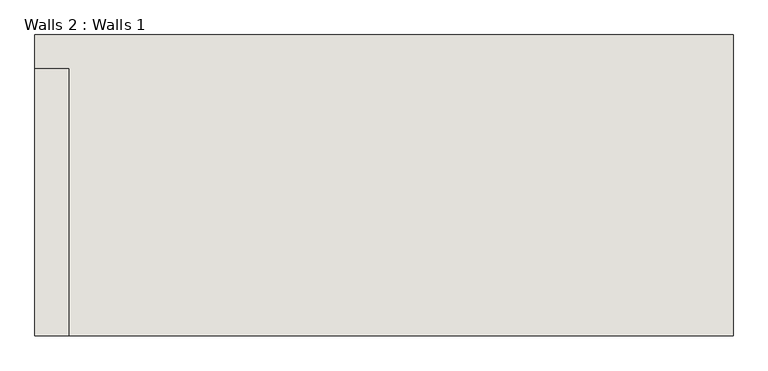
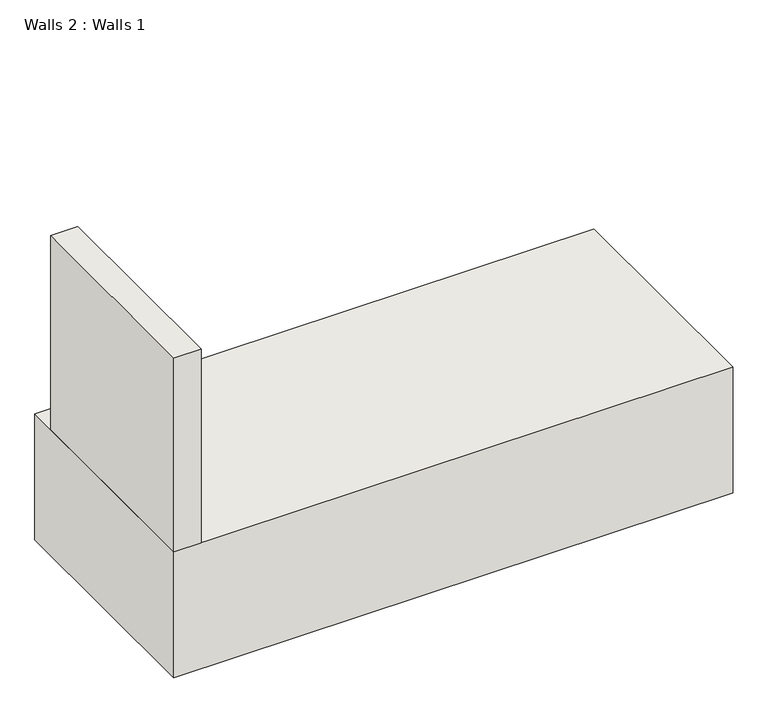
"""IFC4 building model written with IfcOpenShell, lengths in millimetres: wall geometry, Walls 2 : Walls 1."""

from ifc_helpers import new_model, si_unit, frame, origin, place, context, project, spatial, polyline, outline, extrude, source, transform, mapped, element, save


def walls_2_walls_1_41e9462b(model_context):
    return source(origin(), model_context, "Body", "SweptSolid", [
        extrude(outline(polyline([(-4528.4620963, -3412.0885822), (-4528.4620963, -5013.5705746), (-4731.6620963, -5013.5705746), (-4731.6620963, -3412.0885822), (-4528.4620963, -3412.0885822)])), frame((0.0, 0.0, 4959.465177), z_axis=(0.0, 0.0, 1.0), x_axis=(1.0, 0.0, 0.0)), (0.0, 0.0, 1.0), 1539.0744174),
        extrude(outline(polyline([(-540.6620963, -5013.5705746), (-4731.6620963, -5013.5705746), (-4731.6620963, -3208.8885822), (-540.6620963, -3208.8885822), (-540.6620963, -5013.5705746)])), frame((0.0, 0.0, 3962.4), z_axis=(0.0, 0.0, 1.0), x_axis=(1.0, 0.0, 0.0)), (0.0, 0.0, 1.0), 997.065177),
    ])


if __name__ == "__main__":
    model = new_model("IFC4")
    model_context = context("Model", 3, world=origin())
    ifc_project = project(units=[si_unit("LENGTHUNIT", "METRE", prefix="MILLI")], contexts=[model_context])
    site = spatial("IfcSite", under=ifc_project)
    building = spatial("IfcBuilding", under=site)
    placement = place(None, origin())
    walls_2_walls_1_shape = walls_2_walls_1_41e9462b(model_context)
    element("IfcWall", 1, ObjectType="Walls 2 : Walls 1", at=placement, inside=building, context=model_context, shape_type="MappedRepresentation", body=[
        mapped(walls_2_walls_1_shape, transform((0.0, 0.0, 0.0), x_axis=(1.0, 0.0, 0.0), y_axis=(0.0, 1.0, 0.0), z_axis=(0.0, 0.0, 1.0))),
    ])
    save(model, "model.ifc")

# Revit data of these elements
# Element 1 (IfcWall, "Walls 2 : Walls 1")
#   Materials on its faces: "Default Wall"
# Materials
#   "Default Wall": colour RGB 128 128 128, transparency 0
